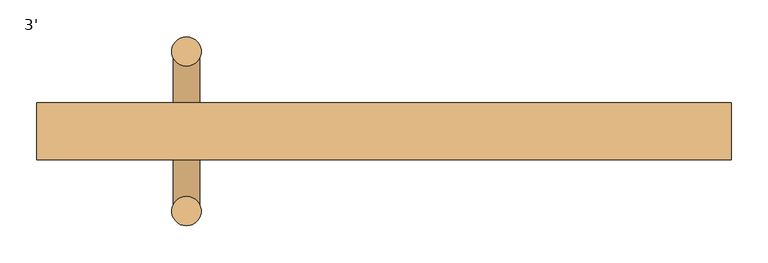
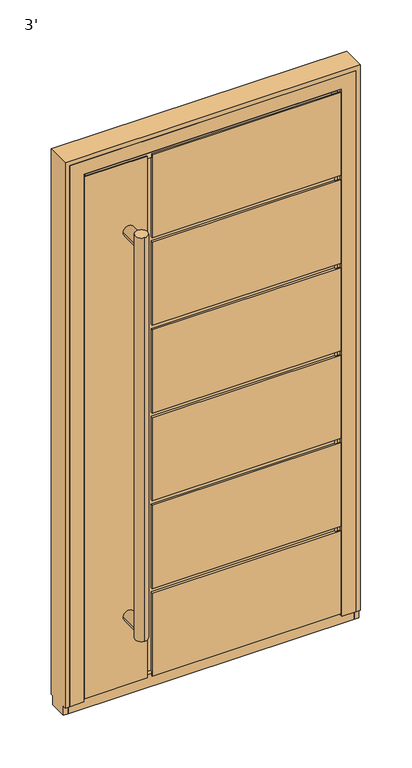
"""IFC4 building model written with IfcOpenShell, lengths in millimetres: door geometry, 3'."""

from ifc_helpers import new_model, si_unit, point, frame, frame_2d, origin, place, context, project, spatial, circle_curve, trimmed, segment, composite_curve, outline, extrude, faceted_brep, source, transform, mapped, element, save


def door_3_44036f4b(model_context):
    return source(origin(), model_context, "Body", "SolidModel", [
        extrude(outline(composite_curve([segment(trimmed(circle_curve(frame_2d((-268.65, 90.8003001)), 20.0), [point((-268.65, 70.8003001))], [point((-268.65, 110.8003001))], False, "CARTESIAN"), True, "CONTINUOUS"), segment(trimmed(circle_curve(frame_2d((-268.65, 90.8003001)), 20.0), [point((-268.65, 110.8003001))], [point((-268.65, 70.8003001))], False, "CARTESIAN"), True, "CONTINUOUS")], self_intersect=False)), frame((0.0, 0.0, 210.0000003), z_axis=(0.0, 0.0, 1.0), x_axis=(1.0, 0.0, 0.0)), (0.0, 0.0, 1.0), 1363.8),
        extrude(outline(composite_curve([segment(trimmed(circle_curve(frame_2d((-268.65, -126.2003001)), 20.0), [point((-268.65, -146.2003001))], [point((-268.65, -106.2003001))], False, "CARTESIAN"), True, "CONTINUOUS"), segment(trimmed(circle_curve(frame_2d((-268.65, -126.2003001)), 20.0), [point((-268.65, -106.2003001))], [point((-268.65, -146.2003001))], False, "CARTESIAN"), True, "CONTINUOUS")], self_intersect=False)), frame((0.0, 0.0, 210.0000003), z_axis=(0.0, 0.0, 1.0), x_axis=(1.0, 0.0, 0.0)), (0.0, 0.0, 1.0), 1363.8),
        extrude(outline(composite_curve([segment(trimmed(circle_curve(frame_2d((241.9000003, -268.65)), 18.0), [point((241.9000003, -286.65))], [point((241.9000003, -250.65))], False, "CARTESIAN"), True, "CONTINUOUS"), segment(trimmed(circle_curve(frame_2d((241.9000003, -268.65)), 18.0), [point((241.9000003, -250.65))], [point((241.9000003, -286.65))], False, "CARTESIAN"), True, "CONTINUOUS")], self_intersect=False)), frame((0.0, -126.2, 0.0), z_axis=(0.0, 1.0, 0.0), x_axis=(0.0, 0.0, 1.0)), (0.0, 0.0, 1.0), 217.0),
        extrude(outline(composite_curve([segment(trimmed(circle_curve(frame_2d((1541.9000003, -268.65)), 18.0), [point((1541.9000003, -286.65))], [point((1541.9000003, -250.65))], False, "CARTESIAN"), True, "CONTINUOUS"), segment(trimmed(circle_curve(frame_2d((1541.9000003, -268.65)), 18.0), [point((1541.9000003, -250.65))], [point((1541.9000003, -286.65))], False, "CARTESIAN"), True, "CONTINUOUS")], self_intersect=False)), frame((0.0, -126.2, 0.0), z_axis=(0.0, 1.0, 0.0), x_axis=(0.0, 0.0, 1.0)), (0.0, 0.0, 1.0), 217.0),
        faceted_brep([(-193.65, 13.8, 306.466667), (383.65, 13.8, 306.466667), (383.65, 13.8, 291.466667), (-193.65, 13.8, 291.466667), (-193.65, 13.8, 35.0), (-208.65, 13.8, 35.0), (-208.65, 13.8, 1748.8000003), (-193.65, 13.8, 1748.8000003), (-193.65, 13.8, 1492.3333337), (383.65, 13.8, 1492.3333337), (383.65, 13.8, 1477.3333337), (-193.65, 13.8, 1477.3333337), (-193.65, 13.8, 1195.866667), (383.65, 13.8, 1195.866667), (383.65, 13.8, 1180.866667), (-193.65, 13.8, 1180.866667), (-193.65, 13.8, 899.4000004), (383.65, 13.8, 899.4000004), (383.65, 13.8, 884.4000004), (-193.65, 13.8, 884.4000004), (-193.65, 13.8, 602.9333337), (383.65, 13.8, 602.9333337), (383.65, 13.8, 587.9333337), (-193.65, 13.8, 587.9333337), (-193.65, 20.8, 587.9333337), (-193.65, 20.8, 306.466667), (383.65, 20.8, 587.9333337), (383.65, 11.7997698, 1748.8000003), (383.65, 11.7997698, 35.0), (383.65, 18.8020472, 35.0), (383.65, 18.8020472, 24.0), (383.65, 20.8, 24.0), (383.65, 20.8, 291.466667), (383.65, 20.8, 306.466667), (383.65, 20.8, 602.9333337), (383.65, 20.8, 884.4000004), (383.65, 20.8, 899.4000004), (383.65, 20.8, 1180.866667), (383.65, 20.8, 1195.866667), (383.65, 20.8, 1477.3333337), (383.65, 20.8, 1492.3333337), (383.65, 20.8, 1748.8000003), (-193.65, 20.8, 602.9333337), (-193.65, 20.8, 884.4000004), (-193.65, 20.8, 899.4000004), (-193.65, 20.8, 1180.866667), (-208.65, 18.8020472, 35.0), (-208.65, 18.8020472, 24.0), (-208.65, 20.8, 24.0), (-208.65, 20.8, 1748.8000003), (-383.65, 11.7997698, 35.0), (-383.65, 18.8020472, 35.0), (-193.65, 18.8020472, 35.0), (-193.65, 20.8, 291.466667), (-193.65, 20.8, 24.0), (-193.65, 18.8020472, 24.0), (-383.65, 18.8020472, 24.0), (-383.65, 20.8, 24.0), (-383.65, 20.8, 1748.8000003), (-193.65, 20.8, 1195.866667), (-193.65, 20.8, 1477.3333337), (-193.65, 20.8, 1492.3333337), (-193.65, 20.8, 1748.8000003), (408.65, -56.2, 10.0000003), (-193.65, -56.2, 10.0000003), (-193.65, -53.2, 10.0000003), (408.65, -53.2, 10.0000003), (-408.65, -53.2, 10.0000003), (-208.65, -53.2, 10.0000003), (-208.65, -56.2, 10.0000003), (-408.65, -56.2, 10.0000003), (408.65, -56.2, 306.466667), (408.65, -53.2, 306.466667), (408.65, -53.2, 587.9333337), (408.65, -56.2, 587.9333337), (408.65, -56.2, 899.4000004), (408.65, -53.2, 899.4000004), (408.65, -53.2, 1180.866667), (408.65, -56.2, 1180.866667), (408.65, -56.2, 602.9333337), (408.65, -53.2, 602.9333337), (408.65, -53.2, 884.4000004), (408.65, -56.2, 884.4000004), (408.65, -56.2, 1195.866667), (408.65, -53.2, 1195.866667), (408.65, -53.2, 1477.3333337), (408.65, -56.2, 1477.3333337), (408.65, -56.2, 1773.8000003), (408.65, -56.2, 1492.3333337), (408.65, -53.2, 1492.3333337), (408.65, -53.2, 1773.8000003), (408.65, -53.2, 291.466667), (408.65, -56.2, 291.466667), (-193.65, -53.2, 25.5), (393.15, -53.2, 25.5), (393.15, -53.2, 291.466667), (393.15, -53.2, 306.466667), (393.15, -53.2, 587.9333337), (393.15, -53.2, 899.4000004), (393.15, -53.2, 1180.866667), (393.15, -53.2, 602.9333337), (393.15, -53.2, 884.4000004), (-393.15, -53.2, 25.5), (-208.65, -53.2, 25.5), (-408.65, -53.2, 1773.8000003), (-208.65, -53.2, 1773.8000003), (-208.65, -53.2, 1758.3000003), (-393.15, -53.2, 1758.3000003), (393.15, -53.2, 1195.866667), (393.15, -53.2, 1477.3333337), (393.15, -53.2, 1492.3333337), (393.15, -53.2, 1758.3000003), (-193.65, -53.2, 1758.3000003), (-193.65, -53.2, 1773.8000003), (-193.65, -49.2, 291.466667), (-193.65, -49.2, 25.5), (-193.65, -56.2, 291.466667), (-208.65, -56.2, 1773.8000003), (-408.65, -56.2, 1773.8000003), (-193.65, -56.2, 587.9333337), (-193.65, -56.2, 306.466667), (-193.65, -56.2, 1180.866667), (-193.65, -56.2, 899.4000004), (-193.65, -56.2, 884.4000004), (-193.65, -56.2, 602.9333337), (-193.65, -56.2, 1477.3333337), (-193.65, -56.2, 1195.866667), (-193.65, -56.2, 1773.8000003), (-193.65, -56.2, 1492.3333337), (-208.65, -49.2, 1758.3000003), (-208.65, -49.2, 25.5), (-383.65, 11.7997698, 1748.8000003), (393.15, 11.7997698, 1758.3000003), (393.15, 11.7997698, 25.5), (-393.15, 11.7997698, 25.5), (-393.15, 11.7997698, 1758.3000003), (393.15, -49.2, 1492.3333337), (393.15, -49.2, 1477.3333337), (393.15, -49.2, 1195.866667), (393.15, -49.2, 1180.866667), (393.15, -49.2, 899.4000004), (393.15, -49.2, 884.4000004), (393.15, -49.2, 602.9333337), (393.15, -49.2, 587.9333337), (393.15, -49.2, 306.466667), (393.15, -49.2, 291.466667), (-193.65, -49.2, 1477.3333337), (-193.65, -49.2, 1492.3333337), (-193.65, -49.2, 1758.3000003), (-193.65, -49.2, 306.466667), (-193.65, -49.2, 587.9333337), (-193.65, -49.2, 602.9333337), (-193.65, -49.2, 884.4000004), (-193.65, -49.2, 899.4000004), (-193.65, -49.2, 1180.866667), (-193.65, -49.2, 1195.866667)], [[[0, 1, 2, 3, 4, 5, 6, 7, 8, 9, 10, 11, 12, 13, 14, 15, 16, 17, 18, 19, 20, 21, 22, 23]], [[23, 24, 25, 0]], [[23, 22, 26, 24]], [[27, 28, 29, 30, 31, 32, 2, 1, 33, 26, 22, 21, 34, 35, 18, 17, 36, 37, 14, 13, 38, 39, 10, 9, 40, 41]], [[42, 34, 21, 20]], [[19, 43, 42, 20]], [[19, 18, 35, 43]], [[44, 36, 17, 16]], [[15, 45, 44, 16]], [[5, 46, 47, 48, 49, 6]], [[28, 50, 51, 46, 5, 4, 52, 29]], [[53, 54, 55, 52, 4, 3]], [[3, 2, 32, 53]], [[25, 33, 1, 0]], [[29, 52, 55, 30]], [[56, 47, 46, 51]], [[30, 55, 54, 31]], [[57, 48, 47, 56]], [[36, 44, 45, 37]], [[34, 42, 43, 35]], [[33, 25, 24, 26]], [[54, 53, 32, 31]], [[58, 49, 48, 57]], [[38, 59, 60, 39]], [[41, 40, 61, 62]], [[63, 64, 65, 66]], [[67, 68, 69, 70]], [[71, 72, 73, 74]], [[75, 76, 77, 78]], [[79, 80, 81, 82]], [[83, 84, 85, 86]], [[87, 88, 89, 90]], [[66, 91, 92, 63]], [[65, 93, 94, 95, 91, 66]], [[72, 96, 97, 73]], [[76, 98, 99, 77]], [[80, 100, 101, 81]], [[102, 103, 68, 67, 104, 105, 106, 107]], [[84, 108, 109, 85]], [[90, 89, 110, 111, 112, 113]], [[114, 115, 93, 65, 64, 116]], [[70, 69, 117, 118]], [[63, 92, 116, 64]], [[74, 119, 120, 71]], [[78, 121, 122, 75]], [[82, 123, 124, 79]], [[86, 125, 126, 83]], [[87, 127, 128, 88]], [[70, 118, 104, 67]], [[129, 106, 105, 117, 69, 68, 103, 130]], [[58, 57, 56, 51, 50, 131]], [[132, 133, 134, 135], [131, 50, 28, 27]], [[111, 110, 136, 137, 109, 108, 138, 139, 99, 98, 140, 141, 101, 100, 142, 143, 97, 96, 144, 145, 95, 94, 133, 132]], [[94, 93, 115, 130, 103, 102, 134, 133]], [[135, 134, 102, 107]], [[146, 137, 136, 147, 148, 129, 130, 115, 114, 145, 144, 149, 150, 143, 142, 151, 152, 141, 140, 153, 154, 139, 138, 155]], [[153, 122, 121, 154]], [[153, 140, 98, 76, 75, 122]], [[123, 82, 81, 101, 141, 152]], [[151, 124, 123, 152]], [[151, 142, 100, 80, 79, 124]], [[119, 74, 73, 97, 143, 150]], [[149, 120, 119, 150]], [[149, 144, 96, 72, 71, 120]], [[116, 92, 91, 95, 145, 114]], [[15, 14, 37, 45]], [[59, 38, 13, 12]], [[11, 60, 59, 12]], [[11, 10, 39, 60]], [[61, 40, 9, 8]], [[8, 7, 62, 61]], [[125, 86, 85, 109, 137, 146]], [[128, 127, 113, 112, 148, 147]], [[121, 78, 77, 99, 139, 154]], [[155, 138, 108, 84, 83, 126]], [[155, 126, 125, 146]], [[147, 136, 110, 89, 88, 128]], [[90, 113, 127, 87]], [[118, 117, 105, 104]], [[132, 135, 107, 106, 129, 148, 112, 111]], [[27, 41, 62, 7, 6, 49, 58, 131]]]),
        faceted_brep([(-457.2, -56.2, 0.0), (-457.2, -47.1997571, 0.0), (-412.7, -47.1997571, 0.0), (-412.7, -56.2, 0.0), (-403.2, 16.2999958, 0.0), (-403.2, 11.8, 0.0), (-457.2, 11.8, 0.0), (-457.2, 20.8, 0.0), (-387.7, 20.8, 0.0), (-387.7, 16.2999958, 0.0), (457.2, 20.8, 0.0), (457.2, 11.8, 0.0), (403.2, 11.8, 0.0), (403.2, 16.2999958, 0.0), (387.7, 16.2999958, 0.0), (387.7, 20.8, 0.0), (412.7, -47.1997571, 0.0), (457.2, -47.1997571, 0.0), (457.2, -56.2, 0.0), (412.7, -56.2, 0.0), (-457.2, 11.8, -30.0), (-457.2, -47.1997571, -30.0), (-457.2, -56.2, 1828.8), (-457.2, 20.8, 1828.8), (-412.7, -56.2, 1784.3), (412.7, -56.2, 1784.3), (457.2, -56.2, 1828.8), (457.2, 20.8, 1828.8), (457.2, -47.1997571, -30.0), (457.2, 11.8, -30.0), (387.7, 20.8, 1759.3), (-387.7, 20.8, 1759.3), (-403.2, -47.2, 1774.8), (-403.2, -47.2, 14.5), (-403.2, 11.8, 14.5), (-403.2, 16.2999958, 1774.8), (403.2, 16.2999958, 1774.8), (403.2, -47.2, 1774.8), (403.2, 11.8, 14.5), (403.2, -47.2, 14.5), (-412.7, -47.2, 1784.3), (412.7, -47.2, 1784.3), (-387.7, 16.2999958, 1759.3), (387.7, 16.2999958, 1759.3)], [[[0, 1, 2, 3]], [[4, 5, 6, 7, 8, 9]], [[10, 11, 12, 13, 14, 15]], [[16, 17, 18, 19]], [[7, 6, 20, 21, 1, 0, 22, 23]], [[3, 24, 25, 19, 18, 26, 22, 0]], [[22, 26, 27, 23]], [[18, 17, 28, 29, 11, 10, 27, 26]], [[7, 23, 27, 10, 15, 30, 31, 8]], [[32, 33, 34, 5, 4, 35]], [[35, 36, 37, 32]], [[36, 13, 12, 38, 39, 37]], [[40, 24, 3, 2]], [[16, 41, 40, 2, 1, 21, 28, 17], [37, 39, 33, 32]], [[9, 42, 43, 14, 13, 36, 35, 4]], [[8, 31, 42, 9]], [[24, 40, 41, 25]], [[30, 43, 42, 31]], [[19, 25, 41, 16]], [[14, 43, 30, 15]], [[20, 6, 5, 34, 38, 12, 11, 29]], [[39, 38, 34, 33]], [[20, 29, 28, 21]]]),
        faceted_brep([(-457.2, -47.2, -30.0), (-472.2, -47.2, -30.0), (-472.2, 11.8, -30.0), (-457.2, 11.8, -30.0), (-457.2, -56.2, 1828.8), (-457.2, -56.2, 0.0), (-457.2, -47.2, 0.0), (-457.2, 11.8, 0.0), (-457.2, 20.8, 0.0), (-457.2, 20.8, 1828.8), (-472.2, 11.8, 0.0), (472.2, 11.8, 0.0), (472.2, 11.8, -30.0), (457.2, 11.8, -30.0), (457.2, 11.8, 0.0), (-472.2, 20.8, 1843.8), (-472.2, 20.8, 0.0), (-472.2, -47.2, 0.0), (-472.2, -56.2, 0.0), (-472.2, -56.2, 1843.8), (457.2, -47.2, 0.0), (457.2, -47.2, -30.0), (472.2, -47.2, -30.0), (472.2, -47.2, 0.0), (457.2, 20.8, 1828.8), (457.2, 20.8, 0.0), (457.2, -56.2, 0.0), (457.2, -56.2, 1828.8), (472.2, -56.2, 0.0), (472.2, -56.2, 1843.8), (472.2, 20.8, 0.0), (472.2, 20.8, 1843.8)], [[[0, 1, 2, 3]], [[4, 5, 6, 0, 3, 7, 8, 9]], [[7, 3, 2, 10]], [[11, 12, 13, 14]], [[15, 16, 10, 2, 1, 17, 18, 19]], [[17, 1, 0, 6]], [[20, 21, 22, 23]], [[24, 25, 14, 13, 21, 20, 26, 27]], [[27, 26, 28, 29, 19, 18, 5, 4]], [[6, 5, 18, 17]], [[23, 28, 26, 20]], [[22, 21, 13, 12]], [[10, 16, 8, 7]], [[14, 25, 30, 11]], [[9, 8, 16, 15, 31, 30, 25, 24]], [[29, 28, 23, 22, 12, 11, 30, 31]], [[9, 24, 27, 4]], [[19, 29, 31, 15]]]),
    ])


if __name__ == "__main__":
    model = new_model("IFC4")
    model_context = context("Model", 3, world=origin())
    ifc_project = project(units=[si_unit("LENGTHUNIT", "METRE", prefix="MILLI")], contexts=[model_context])
    site = spatial("IfcSite", under=ifc_project)
    building = spatial("IfcBuilding", under=site)
    placement = place(None, origin())
    door_3_shape = door_3_44036f4b(model_context)
    element("IfcDoor", 1, ObjectType="3'", at=placement, inside=building, context=model_context, shape_type="MappedRepresentation", body=[
        mapped(door_3_shape, transform((0.0, 0.0, 0.0), x_axis=(1.0, 0.0, 0.0), y_axis=(0.0, 1.0, 0.0), z_axis=(0.0, 0.0, 1.0))),
    ])
    save(model, "model.ifc")

# Revit data of these elements
# Type "3'"
#   Type Mark = "41"
#   Water resistance = "up to Class E900, EN 12208:2001"
#   Uniclass2015Version = "v1.21"
#   Uniclass2015Reference = "Ss_25_30_20_30"
#   Uniclass2015Description = "Frame and door leaf system"
#   URL = "www.aluprof.com"
#   Type IFC Predefined Type = "USERDEFINED"
#   Right-hand / Left-hand door [instance default] = ""
#   Resistance to wind load = "up to Class C5/B5, EN 12210:2001"
#   Insert type = "ST"
#   Hardware [instance default] = ""
#   Product page = "https://aluprof.com/en/architects/offer/window-and-door-systems/panel-doors#visualisation"
#   Operation = "SinglePanelOutwardOpening"
#   Opening type = "Outward"
#   NBSReference = "25-50-20/125"
#   NBSDescription = "Frame and door leaf system"
#   Important = "The actual acceptable construction dimensions are dependent on the selection of profiles and hardware, glazing type, construction weight and the construction’s operating conditions. These should be determined by a suitably qualified person, and using ALUPROF’s calculation software"
#   IfcExportType = "USERDEFINED"
#   IfcExportAs = "IfcDoorType"
#   Handle type [instance default] = ""
#   Manufacturer = "ALUPROF SA"
#   Export Type to IFC As = "IfcDoorType"
#   Door sill type [instance default] = ""
#   Description = "External single-leaf panel door outward opening"
#   Model = "MB-86 ST Panel Door AD07"
#   Content of the recyclate in the material = "69.2%"
#   COBie.Type.WarrantyDurationParts = ""
#   COBie.Type.Name = ""
#   COBie.Type.Manufacturer = "ALUPROF SA"
#   COBie.Space.Name = ""
#   COBie.Floor.Name = ""
#   COBie.Facility.Name = ""
#   COBie.CreatedOn = ""
#   COBie.Component.WarrantyStartDate = ""
#   COBie.Component.Name = "MB-86 ST Panel Door AD07"
#   Burglar resistance = "RC2"
#   Air permeability = "up to Class 4, EN 12207:2001"
#   Width of the active leaf = 2' - 8.17717"
#   Placement in wall = 0' - 0.7874"
#   Thickness = 0' - 3.0315"
#   Height of the opening sash = 5' - 9.44094"
#   Handle Offset = 3' - 5.33858"
#   Rough Height = 6' - 2.40945"
#   Rough Width = 3' - 1.1811"
#   Height = 6' - 0"
#   Width = 3' - 0"
#   Construction depth = 0' - 3.0315"
#   Clear opening width = 2' - 3.94882"
#   Clear opening height = 5' - 8.47638"
#   Height of the array = 0' - 11.08136"
#   Schedule No. [instance default] = 1
#   Handrail [instance default] = yes
#   IsExternal = yes
#   Handle [instance default] = no
#   Door closer [instance default] = no
#   Function = 1
#   COBie.Type = yes
#   COBie = yes
#   Access control [instance default] = no
#   Panel = element 361060
#   Wall Closure = (empty or 0)
